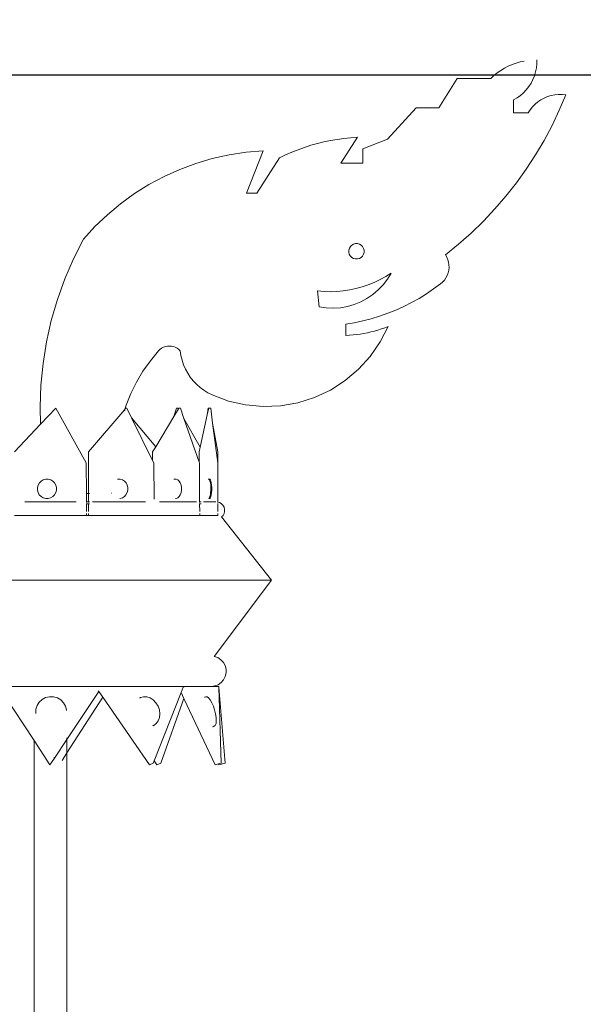
# Model space of a CAD drawing. Units: millimetres. Extents: x 7894 to 8038, y 6851 to 6951.
# Tile 11 of 49: x 7976.35 to 7978.394, y 6875.21 to 6878.784. Entities that reach past the tile are written whole.
import ezdxf

# ---------------------------------------------------------------- set-up
doc = ezdxf.new("R2010")
doc.units = ezdxf.units.MM
for name, color, linetype, lineweight in [('A-ANNO-DIMS', 2, 'Continuous', 18), ('A-FURN-ACCS', 8, 'Continuous', 13), ('A-FURN-SHLF', 7, 'Continuous', 30)]:
    doc.layers.add(name, color=color, linetype=linetype, lineweight=lineweight)
doc.styles.get("Standard").update_dxf_attribs({"font": 'arial.ttf'})
doc.dimstyles.new('ISO-25', dxfattribs={"dimtxt": 1, "dimasz": 1, "dimexe": 1.25, "dimexo": 0.625, "dimtad": 1, "dimdec": 0, "dimlunit": 4, "dimtxsty": 'Standard', "dimcen": 2.5, "dimclrt": 1, "dimadec": 0, "dimazin": 0, "dimtfac": 1, "dimtdec": 0, "dimtmove": 0, "dimatfit": 3, "dimfxl": 1, "dimarcsym": 0})

# ---------------------------------------------------------------- blocks, each defined once
blk = doc.blocks.new('*D36')
at = {"layer": 'A-ANNO-DIMS', "color": 0, "lineweight": -2, "transparency": 16777216}
for p, q in [((7980.8359, 6877.9586), (7980.8359, 6858.5122)), ((7944.4866, 6864.4359), (7944.4866, 6858.5122)), ((7945.4866, 6859.7622), (7979.8359, 6859.7622))]:
    blk.add_line(p, q, dxfattribs=at)
at = {"layer": 'A-ANNO-DIMS', "color": 0, "transparency": 16777216}
for points in [[(7945.4866, 6859.9288), (7945.4866, 6859.5955), (7944.4866, 6859.7622)], [(7979.8359, 6859.9288), (7979.8359, 6859.5955), (7980.8359, 6859.7622)]]:
    blk.add_solid(points, dxfattribs=at)
at = {"layer": 'Defpoints', "color": 0, "transparency": 16777216}
for p in [(7980.8359, 6878.5836), (7944.4866, 6865.0609), (7980.8359, 6859.7622)]:
    blk.add_point(p, dxfattribs=at)
at = {"layer": 'A-ANNO-DIMS', "color": 1, "transparency": 16777216, "insert": (7962.6613, 6860.9046), "char_height": 1, "attachment_point": 5}
blk.add_mtext('3\'-0 1/2"', dxfattribs=at)
blk = doc.blocks.new('*D39')
at = {"layer": 'A-ANNO-DIMS', "color": 0, "lineweight": -2, "transparency": 16777216}
for p, q in [((7982.6834, 6874.8578), (7982.6834, 6879.7661)), ((7964.1574, 6873.8578), (7983.9334, 6873.8578)), ((7982.6834, 6872.9028), (7982.6834, 6873.8578)), ((7981.4609, 6872.9028), (7983.9334, 6872.9028)), ((7982.6834, 6871.9028), (7982.6834, 6870.9028))]:
    blk.add_line(p, q, dxfattribs=at)
at = {"layer": 'A-ANNO-DIMS', "color": 0, "transparency": 16777216}
for points in [[(7982.5168, 6874.8578), (7982.8501, 6874.8578), (7982.6834, 6873.8578)], [(7982.5168, 6871.9028), (7982.8501, 6871.9028), (7982.6834, 6872.9028)]]:
    blk.add_solid(points, dxfattribs=at)
at = {"layer": 'Defpoints', "color": 0, "transparency": 16777216}
for p in [(7963.5324, 6873.8578), (7982.6834, 6873.8578), (7980.8359, 6872.9028)]:
    blk.add_point(p, dxfattribs=at)
at = {"layer": 'A-ANNO-DIMS', "color": 1, "transparency": 16777216, "insert": (7981.5479, 6877.8119), "char_height": 1, "attachment_point": 5, "rotation": 90}
blk.add_mtext('0\'-1"', dxfattribs=at)
blk = doc.blocks.new('*D40')
at = {"layer": 'A-ANNO-DIMS', "color": 0, "lineweight": -2, "transparency": 16777216}
for p, q in [((7982.6834, 6878.5836), (7982.6834, 6885.822)), ((7981.4609, 6878.5836), (7983.9334, 6878.5836)), ((7982.6834, 6874.8578), (7982.6834, 6877.5836)), ((7964.1574, 6873.8578), (7983.9334, 6873.8578))]:
    blk.add_line(p, q, dxfattribs=at)
at = {"layer": 'A-ANNO-DIMS', "color": 0, "transparency": 16777216}
for points in [[(7982.5168, 6877.5836), (7982.8501, 6877.5836), (7982.6834, 6878.5836)], [(7982.5168, 6874.8578), (7982.8501, 6874.8578), (7982.6834, 6873.8578)]]:
    blk.add_solid(points, dxfattribs=at)
at = {"layer": 'Defpoints', "color": 0, "transparency": 16777216}
for p in [(7980.8359, 6878.5836), (7982.6834, 6878.5836), (7963.5324, 6873.8578)]:
    blk.add_point(p, dxfattribs=at)
at = {"layer": 'A-ANNO-DIMS', "color": 1, "transparency": 16777216, "insert": (7981.5414, 6882.7028), "char_height": 1, "attachment_point": 5, "rotation": 90}
blk.add_mtext('0\'-4 1/2"', dxfattribs=at)

msp = doc.modelspace()

# ---------------------------------------------------------------- linework, layer by layer
at = {"layer": 'A-FURN-ACCS'}
for p, q in [((7978.1353, 6878.6211, 2.197), (7978.1497, 6878.6264, 2.197)), ((7978.1497, 6878.6264, 2.197), (7978.1645, 6878.6307, 2.197)), ((7978.1645, 6878.6307, 2.197), (7978.1795, 6878.6341, 2.197)), ((7978.2253, 6878.6385, 2.197), (7978.2252, 6878.6237, 2.197)), ((7978.0697, 6878.5816, 2.197), (7978.0818, 6878.5912, 2.197)), ((7978.0818, 6878.5912, 2.197), (7978.0944, 6878.5999, 2.197)), ((7978.0944, 6878.5999, 2.197), (7978.1076, 6878.6079, 2.197)), ((7978.1076, 6878.6079, 2.197), (7978.1212, 6878.6149, 2.197)), ((7978.1212, 6878.6149, 2.197), (7978.1353, 6878.6211, 2.197)), ((7978.2208, 6878.5946, 2.197), (7978.2166, 6878.5804, 2.197)), ((7978.2237, 6878.6091, 2.197), (7978.2208, 6878.5946, 2.197)), ((7978.2252, 6878.6237, 2.197), (7978.2237, 6878.6091, 2.197)), ((7977.8697, 6878.4643, 2.197), (7977.9359, 6878.5713, 2.197)), ((7977.9359, 6878.5713, 2.197), (7978.0583, 6878.5713, 2.197)), ((7978.0583, 6878.5713, 2.197), (7978.0697, 6878.5816, 2.197)), ((7978.2042, 6878.5537, 2.197), (7978.1962, 6878.5413, 2.197)), ((7978.211, 6878.5668, 2.197), (7978.2042, 6878.5537, 2.197)), ((7978.2166, 6878.5804, 2.197), (7978.211, 6878.5668, 2.197)), ((7978.1768, 6878.5191, 2.197), (7978.1656, 6878.5095, 2.197)), ((7978.187, 6878.5297, 2.197), (7978.1768, 6878.5191, 2.197)), ((7978.1962, 6878.5413, 2.197), (7978.187, 6878.5297, 2.197)), ((7978.1536, 6878.5009, 2.197), (7978.1408, 6878.4936, 2.197)), ((7978.1408, 6878.4936, 2.197), (7978.1408, 6878.4464, 2.197)), ((7978.1656, 6878.5095, 2.197), (7978.1536, 6878.5009, 2.197)), ((7978.2187, 6878.4773, 2.197), (7978.2291, 6878.4858, 2.197)), ((7978.2291, 6878.4858, 2.197), (7978.2402, 6878.4933, 2.197)), ((7978.2402, 6878.4933, 2.197), (7978.252, 6878.4997, 2.197)), ((7978.252, 6878.4997, 2.197), (7978.2644, 6878.5048, 2.197)), ((7978.2644, 6878.5048, 2.197), (7978.2772, 6878.5088, 2.197)), ((7978.2772, 6878.5088, 2.197), (7978.2903, 6878.5115, 2.197)), ((7978.2903, 6878.5115, 2.197), (7978.3036, 6878.513, 2.197)), ((7978.3036, 6878.513, 2.197), (7978.317, 6878.5131, 2.197)), ((7978.3304, 6878.5119, 2.197), (7978.3066, 6878.4554, 2.197)), ((7978.317, 6878.5131, 2.197), (7978.3304, 6878.5119, 2.197)), ((7977.6836, 6878.3509, 2.197), (7977.7876, 6878.4643, 2.197)), ((7977.7876, 6878.4643, 2.197), (7977.8697, 6878.4643, 2.197)), ((7978.1408, 6878.4464, 2.197), (7978.1932, 6878.4464, 2.197)), ((7978.1932, 6878.4464, 2.197), (7978.2007, 6878.4575, 2.197)), ((7978.2007, 6878.4575, 2.197), (7978.2092, 6878.4678, 2.197)), ((7978.2092, 6878.4678, 2.197), (7978.2187, 6878.4773, 2.197)), ((7978.3066, 6878.4554, 2.197), (7978.2803, 6878.4, 2.197)), ((7978.2803, 6878.4, 2.197), (7978.2515, 6878.3459, 2.197)), ((7977.4292, 6878.3349, 2.197), (7977.453, 6878.3408, 2.197)), ((7977.453, 6878.3408, 2.197), (7977.477, 6878.3458, 2.197)), ((7977.477, 6878.3458, 2.197), (7977.5011, 6878.3499, 2.197)), ((7977.5011, 6878.3499, 2.197), (7977.5254, 6878.3532, 2.197)), ((7977.5743, 6878.3572, 2.197), (7977.5139, 6878.263, 2.197)), ((7977.5254, 6878.3532, 2.197), (7977.5498, 6878.3556, 2.197)), ((7977.5498, 6878.3556, 2.197), (7977.5743, 6878.3572, 2.197)), ((7977.5943, 6878.3154, 2.197), (7977.6836, 6878.3509, 2.197)), ((7978.2515, 6878.3459, 2.197), (7978.2204, 6878.2931, 2.197)), ((7977.109, 6878.294, 2.197), (7977.1706, 6878.3034, 2.197)), ((7977.1706, 6878.3034, 2.197), (7977.2326, 6878.3087, 2.197)), ((7977.2326, 6878.3087, 2.197), (7977.1717, 6878.1542, 2.197)), ((7977.3142, 6878.2931, 2.197), (7977.3365, 6878.3031, 2.197)), ((7977.3365, 6878.3031, 2.197), (7977.3592, 6878.3123, 2.197)), ((7977.3592, 6878.3123, 2.197), (7977.3823, 6878.3206, 2.197)), ((7977.3823, 6878.3206, 2.197), (7977.4056, 6878.3282, 2.197)), ((7977.4056, 6878.3282, 2.197), (7977.4292, 6878.3349, 2.197)), ((7977.5943, 6878.263, 2.197), (7977.5943, 6878.3154, 2.197)), ((7976.9885, 6878.2626, 2.197), (7977.0482, 6878.2803, 2.197)), ((7977.0482, 6878.2803, 2.197), (7977.109, 6878.294, 2.197)), ((7977.2101, 6878.1542, 2.197), (7977.2921, 6878.2823, 2.197)), ((7977.2921, 6878.2823, 2.197), (7977.3142, 6878.2931, 2.197)), ((7978.2204, 6878.2931, 2.197), (7978.1869, 6878.2417, 2.197)), ((7976.8733, 6878.2153, 2.197), (7976.9301, 6878.2409, 2.197)), ((7976.9301, 6878.2409, 2.197), (7976.9885, 6878.2626, 2.197)), ((7977.5139, 6878.263, 2.197), (7977.5943, 6878.263, 2.197)), ((7978.1869, 6878.2417, 2.197), (7978.1512, 6878.1919, 2.197)), ((7976.8184, 6878.1858, 2.197), (7976.8733, 6878.2153, 2.197)), ((7976.7657, 6878.1527, 2.197), (7976.8184, 6878.1858, 2.197)), ((7978.1512, 6878.1919, 2.197), (7978.1132, 6878.1437, 2.197)), ((7976.7153, 6878.1161, 2.197), (7976.7657, 6878.1527, 2.197)), ((7977.1717, 6878.1542, 2.197), (7977.2101, 6878.1542, 2.197)), ((7978.1132, 6878.1437, 2.197), (7978.0732, 6878.0972, 2.197)), ((7976.6675, 6878.0762, 2.197), (7976.7153, 6878.1161, 2.197)), ((7978.0732, 6878.0972, 2.197), (7978.0312, 6878.0526, 2.197)), ((7976.6225, 6878.0331, 2.197), (7976.6675, 6878.0762, 2.197)), ((7976.5805, 6877.987, 2.197), (7976.6225, 6878.0331, 2.197)), ((7978.0312, 6878.0526, 2.197), (7977.9872, 6878.0099, 2.197)), ((7976.5805, 6877.987, 2.197), (7976.5447, 6877.9162, 2.197)), ((7977.9872, 6878.0099, 2.197), (7977.9413, 6877.9692, 2.197)), ((7977.5432, 6877.9399, 2.197), (7977.5433, 6877.9472, 2.197)), ((7977.5433, 6877.9472, 2.197), (7977.5452, 6877.9543, 2.197)), ((7977.5452, 6877.9543, 2.197), (7977.5489, 6877.9606, 2.197)), ((7977.5489, 6877.9606, 2.197), (7977.5541, 6877.9657, 2.197)), ((7977.5541, 6877.9657, 2.197), (7977.5604, 6877.9693, 2.197)), ((7977.5604, 6877.9693, 2.197), (7977.5675, 6877.9712, 2.197)), ((7977.5675, 6877.9712, 2.197), (7977.5748, 6877.9712, 2.197)), ((7977.5748, 6877.9712, 2.197), (7977.5818, 6877.9692, 2.197)), ((7977.5818, 6877.9692, 2.197), (7977.5881, 6877.9656, 2.197)), ((7977.5881, 6877.9656, 2.197), (7977.5933, 6877.9604, 2.197)), ((7977.5933, 6877.9604, 2.197), (7977.5969, 6877.954, 2.197)), ((7977.5969, 6877.954, 2.197), (7977.5987, 6877.947, 2.197)), ((7977.5987, 6877.947, 2.197), (7977.5987, 6877.9397, 2.197)), ((7977.9413, 6877.9692, 2.197), (7977.8937, 6877.9306, 2.197)), ((7976.5447, 6877.9162, 2.197), (7976.5133, 6877.8432, 2.197)), ((7977.5451, 6877.9329, 2.197), (7977.5432, 6877.9399, 2.197)), ((7977.5487, 6877.9265, 2.197), (7977.5451, 6877.9329, 2.197)), ((7977.5538, 6877.9214, 2.197), (7977.5487, 6877.9265, 2.197)), ((7977.5601, 6877.9177, 2.197), (7977.5538, 6877.9214, 2.197)), ((7977.5672, 6877.9158, 2.197), (7977.5601, 6877.9177, 2.197)), ((7977.5745, 6877.9157, 2.197), (7977.5672, 6877.9158, 2.197)), ((7977.5815, 6877.9176, 2.197), (7977.5745, 6877.9157, 2.197)), ((7977.5879, 6877.9212, 2.197), (7977.5815, 6877.9176, 2.197)), ((7977.5931, 6877.9263, 2.197), (7977.5879, 6877.9212, 2.197)), ((7977.5968, 6877.9326, 2.197), (7977.5931, 6877.9263, 2.197)), ((7977.5987, 6877.9397, 2.197), (7977.5968, 6877.9326, 2.197)), ((7977.8937, 6877.9306, 2.197), (7977.8985, 6877.9222, 2.197)), ((7977.8985, 6877.9222, 2.197), (7977.9023, 6877.9131, 2.197)), ((7977.9023, 6877.9131, 2.197), (7977.9049, 6877.9037, 2.197)), ((7977.9056, 6877.8746, 2.197), (7977.9034, 6877.8651, 2.197)), ((7977.9049, 6877.9037, 2.197), (7977.9064, 6877.8941, 2.197)), ((7977.9066, 6877.8843, 2.197), (7977.9056, 6877.8746, 2.197)), ((7977.9064, 6877.8941, 2.197), (7977.9066, 6877.8843, 2.197)), ((7976.5133, 6877.8432, 2.197), (7976.4865, 6877.7684, 2.197)), ((7977.6566, 6877.8406, 2.197), (7977.6355, 6877.8306, 2.197)), ((7977.677, 6877.8518, 2.197), (7977.6566, 6877.8406, 2.197)), ((7977.6833, 6877.8424, 2.197), (7977.6676, 6877.822, 2.197)), ((7977.6968, 6877.8643, 2.197), (7977.677, 6877.8518, 2.197)), ((7977.6968, 6877.8643, 2.197), (7977.6833, 6877.8424, 2.197)), ((7977.89, 6877.8392, 2.197), (7977.8835, 6877.8319, 2.197)), ((7977.8955, 6877.8472, 2.197), (7977.89, 6877.8392, 2.197)), ((7977.9, 6877.8559, 2.197), (7977.8955, 6877.8472, 2.197)), ((7977.9034, 6877.8651, 2.197), (7977.9, 6877.8559, 2.197)), ((7977.5464, 6877.8033, 2.197), (7977.5233, 6877.7998, 2.197)), ((7977.5692, 6877.8081, 2.197), (7977.5464, 6877.8033, 2.197)), ((7977.5917, 6877.8143, 2.197), (7977.5692, 6877.8081, 2.197)), ((7977.6138, 6877.8218, 2.197), (7977.5917, 6877.8143, 2.197)), ((7977.6355, 6877.8306, 2.197), (7977.6138, 6877.8218, 2.197)), ((7977.6499, 6877.8034, 2.197), (7977.6303, 6877.7868, 2.197)), ((7977.6676, 6877.822, 2.197), (7977.6499, 6877.8034, 2.197)), ((7977.8508, 6877.8068, 2.197), (7977.8246, 6877.7892, 2.197)), ((7977.8761, 6877.8255, 2.197), (7977.8508, 6877.8068, 2.197)), ((7977.8835, 6877.8319, 2.197), (7977.8761, 6877.8255, 2.197)), ((7976.4865, 6877.7684, 2.197), (7976.4643, 6877.6922, 2.197)), ((7977.4534, 6877.7975, 2.197), (7977.4301, 6877.7995, 2.197)), ((7977.4301, 6877.7995, 2.197), (7977.4358, 6877.7415, 2.197)), ((7977.4767, 6877.7969, 2.197), (7977.4534, 6877.7975, 2.197)), ((7977.5, 6877.7977, 2.197), (7977.4767, 6877.7969, 2.197)), ((7977.5233, 6877.7998, 2.197), (7977.5, 6877.7977, 2.197)), ((7977.6091, 6877.7723, 2.197), (7977.5864, 6877.7602, 2.197)), ((7977.6303, 6877.7868, 2.197), (7977.6091, 6877.7723, 2.197)), ((7977.7978, 6877.7727, 2.197), (7977.7703, 6877.7573, 2.197)), ((7977.8246, 6877.7892, 2.197), (7977.7978, 6877.7727, 2.197)), ((7977.4613, 6877.7379, 2.197), (7977.4358, 6877.7415, 2.197)), ((7977.487, 6877.737, 2.197), (7977.4613, 6877.7379, 2.197)), ((7977.5126, 6877.7388, 2.197), (7977.487, 6877.737, 2.197)), ((7977.5379, 6877.7433, 2.197), (7977.5126, 6877.7388, 2.197)), ((7977.5626, 6877.7505, 2.197), (7977.5379, 6877.7433, 2.197)), ((7977.5864, 6877.7602, 2.197), (7977.5626, 6877.7505, 2.197)), ((7977.7422, 6877.7432, 2.197), (7977.7135, 6877.7302, 2.197)), ((7977.7703, 6877.7573, 2.197), (7977.7422, 6877.7432, 2.197)), ((7977.6244, 6877.6986, 2.197), (7977.594, 6877.6906, 2.197)), ((7977.6546, 6877.7079, 2.197), (7977.6244, 6877.6986, 2.197)), ((7977.6842, 6877.7184, 2.197), (7977.6546, 6877.7079, 2.197)), ((7977.7135, 6877.7302, 2.197), (7977.6842, 6877.7184, 2.197)), ((7976.4643, 6877.6922, 2.197), (7976.4469, 6877.6147, 2.197)), ((7977.5632, 6877.6839, 2.197), (7977.5322, 6877.6784, 2.197)), ((7977.5322, 6877.6784, 2.197), (7977.5322, 6877.6382, 2.197)), ((7977.594, 6877.6906, 2.197), (7977.5632, 6877.6839, 2.197)), ((7977.6488, 6877.6576, 2.197), (7977.6614, 6877.6617, 2.197)), ((7977.6861, 6877.6709, 2.197), (7977.6571, 6877.6143, 2.197)), ((7977.6614, 6877.6617, 2.197), (7977.6738, 6877.6661, 2.197)), ((7977.6738, 6877.6661, 2.197), (7977.6861, 6877.6709, 2.197)), ((7977.5322, 6877.6382, 2.197), (7977.5453, 6877.6389, 2.197)), ((7977.5453, 6877.6389, 2.197), (7977.5585, 6877.6399, 2.197)), ((7977.5585, 6877.6399, 2.197), (7977.5716, 6877.6412, 2.197)), ((7977.5716, 6877.6412, 2.197), (7977.5846, 6877.643, 2.197)), ((7977.5846, 6877.643, 2.197), (7977.5976, 6877.6452, 2.197)), ((7977.5976, 6877.6452, 2.197), (7977.6106, 6877.6477, 2.197)), ((7977.6106, 6877.6477, 2.197), (7977.6234, 6877.6506, 2.197)), ((7977.6234, 6877.6506, 2.197), (7977.6362, 6877.6539, 2.197)), ((7977.6362, 6877.6539, 2.197), (7977.6488, 6877.6576, 2.197)), ((7976.4469, 6877.6147, 2.197), (7976.4343, 6877.5362, 2.197)), ((7976.8644, 6877.5915, 2.197), (7976.8584, 6877.5872, 2.197)), ((7976.8709, 6877.595, 2.197), (7976.8644, 6877.5915, 2.197)), ((7976.8779, 6877.5975, 2.197), (7976.8709, 6877.595, 2.197)), ((7976.8851, 6877.599, 2.197), (7976.8779, 6877.5975, 2.197)), ((7976.8924, 6877.5996, 2.197), (7976.8851, 6877.599, 2.197)), ((7976.8998, 6877.599, 2.197), (7976.8924, 6877.5996, 2.197)), ((7976.907, 6877.5975, 2.197), (7976.8998, 6877.599, 2.197)), ((7976.914, 6877.595, 2.197), (7976.907, 6877.5975, 2.197)), ((7976.9205, 6877.5915, 2.197), (7976.914, 6877.595, 2.197)), ((7976.9264, 6877.5872, 2.197), (7976.9205, 6877.5915, 2.197)), ((7977.6571, 6877.6143, 2.197), (7977.621, 6877.5621, 2.197)), ((7976.8531, 6877.5821, 2.197), (7976.8235, 6877.5465, 2.197)), ((7976.8584, 6877.5872, 2.197), (7976.8531, 6877.5821, 2.197)), ((7976.9318, 6877.5821, 2.197), (7976.9264, 6877.5872, 2.197)), ((7976.9343, 6877.565, 2.197), (7976.9318, 6877.5821, 2.197)), ((7976.9383, 6877.5483, 2.197), (7976.9343, 6877.565, 2.197)), ((7977.621, 6877.5621, 2.197), (7977.5784, 6877.5151, 2.197)), ((7976.4343, 6877.5362, 2.197), (7976.4266, 6877.4572, 2.197)), ((7976.8235, 6877.5465, 2.197), (7976.7968, 6877.5088, 2.197)), ((7976.9438, 6877.5319, 2.197), (7976.9383, 6877.5483, 2.197)), ((7976.9506, 6877.5161, 2.197), (7976.9438, 6877.5319, 2.197)), ((7976.7968, 6877.5088, 2.197), (7976.7731, 6877.469, 2.197)), ((7976.9588, 6877.501, 2.197), (7976.9506, 6877.5161, 2.197)), ((7976.9683, 6877.4866, 2.197), (7976.9588, 6877.501, 2.197)), ((7976.979, 6877.4731, 2.197), (7976.9683, 6877.4866, 2.197)), ((7977.5784, 6877.5151, 2.197), (7977.5299, 6877.4741, 2.197)), ((7976.4266, 6877.4572, 2.197), (7976.4238, 6877.3778, 2.197)), ((7976.7731, 6877.469, 2.197), (7976.7526, 6877.4275, 2.197)), ((7976.9909, 6877.4606, 2.197), (7976.979, 6877.4731, 2.197)), ((7977.0038, 6877.4492, 2.197), (7976.9909, 6877.4606, 2.197)), ((7977.0176, 6877.4389, 2.197), (7977.0038, 6877.4492, 2.197)), ((7977.5299, 6877.4741, 2.197), (7977.4764, 6877.4399, 2.197)), ((7976.7526, 6877.4275, 2.197), (7976.7355, 6877.3845, 2.197)), ((7977.0323, 6877.4299, 2.197), (7977.0176, 6877.4389, 2.197)), ((7977.0477, 6877.4222, 2.197), (7977.0323, 6877.4299, 2.197)), ((7977.1072, 6877.4001, 2.197), (7977.0477, 6877.4222, 2.197)), ((7977.4189, 6877.413, 2.197), (7977.3583, 6877.3939, 2.197)), ((7977.4764, 6877.4399, 2.197), (7977.4189, 6877.413, 2.197)), ((7976.4238, 6877.3778, 2.197), (7976.4254, 6877.3158, 2.197)), ((7976.4811, 6877.3745, 2.197), (7976.4254, 6877.3158, 2.197)), ((7976.5903, 6877.1753, 2.197), (7976.4811, 6877.3745, 2.197)), ((7976.7355, 6877.3845, 2.197), (7976.7311, 6877.3702, 2.197)), ((7976.7348, 6877.3745, 2.197), (7976.7311, 6877.3702, 2.197)), ((7976.7348, 6877.3745, 2.197), (7976.7379, 6877.3745, 2.197)), ((7976.7552, 6877.3393, 2.197), (7976.7379, 6877.3745, 2.197)), ((7976.9082, 6877.3433, 2.197), (7976.9184, 6877.3745, 2.197)), ((7976.9184, 6877.3745, 2.197), (7976.924, 6877.3745, 2.197)), ((7976.924, 6877.3745, 2.197), (7976.9254, 6877.3721, 2.197)), ((7976.9269, 6877.3745, 2.197), (7976.9254, 6877.3721, 2.197)), ((7976.9269, 6877.3745, 2.197), (7976.9323, 6877.3745, 2.197)), ((7976.9454, 6877.3369, 2.197), (7976.9323, 6877.3745, 2.197)), ((7977.03, 6877.3496, 2.197), (7977.0326, 6877.3745, 2.197)), ((7977.0355, 6877.3745, 2.197), (7977.03, 6877.3496, 2.197)), ((7977.0326, 6877.3745, 2.197), (7977.0355, 6877.3745, 2.197)), ((7977.0355, 6877.3745, 2.197), (7977.0423, 6877.3745, 2.197)), ((7977.0423, 6877.3745, 2.197), (7977.0492, 6877.3201, 2.197)), ((7977.1691, 6877.3861, 2.197), (7977.1072, 6877.4001, 2.197)), ((7977.2324, 6877.3803, 2.197), (7977.1691, 6877.3861, 2.197)), ((7977.2958, 6877.3829, 2.197), (7977.2324, 6877.3803, 2.197)), ((7977.3583, 6877.3939, 2.197), (7977.2958, 6877.3829, 2.197)), ((7976.7307, 6877.3688, 2.197), (7976.5997, 6877.2159, 2.197)), ((7976.7307, 6877.3688, 2.197), (7976.7293, 6877.3645, 2.197)), ((7976.7311, 6877.3702, 2.197), (7976.7307, 6877.3688, 2.197)), ((7976.7307, 6877.3688, 2.197), (7976.7318, 6877.3674, 2.197)), ((7976.7552, 6877.3393, 2.197), (7976.8428, 6877.2342, 2.197)), ((7976.7552, 6877.3393, 2.197), (7976.8318, 6877.1842, 2.197)), ((7976.9082, 6877.3433, 2.197), (7976.8428, 6877.2342, 2.197)), ((7976.9254, 6877.3721, 2.197), (7976.9082, 6877.3433, 2.197)), ((7977.03, 6877.3496, 2.197), (7977.0044, 6877.2329, 2.197)), ((7976.4254, 6877.3158, 2.197), (7976.3309, 6877.2159, 2.197)), ((7976.9454, 6877.3369, 2.197), (7977.0044, 6877.2329, 2.197)), ((7976.9454, 6877.3369, 2.197), (7977.0007, 6877.1778, 2.197)), ((7977.0492, 6877.3201, 2.197), (7977.0679, 6877.2159, 2.197)), ((7977.0676, 6877.1753, 2.197), (7977.0492, 6877.3201, 2.197)), ((7976.8428, 6877.2342, 2.197), (7976.8318, 6877.2159, 2.197)), ((7977.0044, 6877.2329, 2.197), (7977.0007, 6877.2159, 2.197)), ((7976.5997, 6877.2159, 2.197), (7976.5997, 6877.0643, 2.197)), ((7976.8318, 6877.2159, 2.197), (7976.8318, 6877.1842, 2.197)), ((7977.0007, 6877.2159, 2.197), (7977.0007, 6877.1778, 2.197)), ((7977.0679, 6877.2159, 2.197), (7977.0676, 6877.1753, 2.197)), ((7976.5903, 6877.1753, 2.197), (7976.5913, 6877.0642, 2.197)), ((7976.8362, 6877.1753, 2.197), (7976.8318, 6877.1842, 2.197)), ((7976.8362, 6877.1753, 2.197), (7976.8372, 6877.0442, 2.197)), ((7977.0015, 6877.1753, 2.197), (7977.0007, 6877.1778, 2.197)), ((7977.0015, 6877.1753, 2.197), (7977.0023, 6877.0335, 2.197)), ((7977.0676, 6877.1753, 2.197), (7977.0679, 6877.033, 2.197)), ((7976.414, 6877.086, 2.197), (7976.4164, 6877.0948, 2.197)), ((7976.4164, 6877.0948, 2.197), (7976.421, 6877.1027, 2.197)), ((7976.421, 6877.1027, 2.197), (7976.4274, 6877.1091, 2.197)), ((7976.4274, 6877.1091, 2.197), (7976.4353, 6877.1137, 2.197)), ((7976.4353, 6877.1137, 2.197), (7976.4442, 6877.116, 2.197)), ((7976.4442, 6877.116, 2.197), (7976.4533, 6877.116, 2.197)), ((7976.4533, 6877.116, 2.197), (7976.4621, 6877.1136, 2.197)), ((7976.4621, 6877.1136, 2.197), (7976.47, 6877.109, 2.197)), ((7976.47, 6877.109, 2.197), (7976.4764, 6877.1025, 2.197)), ((7976.4764, 6877.1025, 2.197), (7976.481, 6877.0946, 2.197)), ((7976.481, 6877.0946, 2.197), (7976.4833, 6877.0858, 2.197)), ((7976.7047, 6877.116, 2.197), (7976.7062, 6877.116, 2.197)), ((7976.7062, 6877.116, 2.197), (7976.7144, 6877.116, 2.197)), ((7976.7144, 6877.116, 2.197), (7976.7223, 6877.1136, 2.197)), ((7976.7223, 6877.1136, 2.197), (7976.7294, 6877.109, 2.197)), ((7976.7294, 6877.109, 2.197), (7976.7352, 6877.1025, 2.197)), ((7976.7352, 6877.1025, 2.197), (7976.7393, 6877.0946, 2.197)), ((7976.7393, 6877.0946, 2.197), (7976.7414, 6877.0858, 2.197)), ((7976.9089, 6877.116, 2.197), (7976.9117, 6877.116, 2.197)), ((7976.9117, 6877.116, 2.197), (7976.9174, 6877.116, 2.197)), ((7976.9174, 6877.116, 2.197), (7976.923, 6877.1136, 2.197)), ((7976.923, 6877.1136, 2.197), (7976.928, 6877.109, 2.197)), ((7976.928, 6877.109, 2.197), (7976.9321, 6877.1025, 2.197)), ((7976.9321, 6877.1025, 2.197), (7976.935, 6877.0946, 2.197)), ((7976.935, 6877.0946, 2.197), (7976.9364, 6877.0858, 2.197)), ((7977.0337, 6877.116, 2.197), (7977.0358, 6877.116, 2.197)), ((7977.0358, 6877.116, 2.197), (7977.0379, 6877.1136, 2.197)), ((7977.0358, 6877.116, 2.197), (7977.0371, 6877.116, 2.197)), ((7977.0371, 6877.116, 2.197), (7977.0392, 6877.116, 2.197)), ((7977.0379, 6877.1136, 2.197), (7977.0397, 6877.109, 2.197)), ((7977.0392, 6877.116, 2.197), (7977.0413, 6877.1136, 2.197)), ((7977.0397, 6877.109, 2.197), (7977.0412, 6877.1025, 2.197)), ((7977.0412, 6877.1025, 2.197), (7977.0423, 6877.0946, 2.197)), ((7977.0413, 6877.1136, 2.197), (7977.0431, 6877.109, 2.197)), ((7977.0423, 6877.0946, 2.197), (7977.0428, 6877.0858, 2.197)), ((7977.0431, 6877.109, 2.197), (7977.0446, 6877.1025, 2.197)), ((7977.0446, 6877.1025, 2.197), (7977.0457, 6877.0946, 2.197)), ((7977.0457, 6877.0946, 2.197), (7977.0462, 6877.0858, 2.197)), ((7976.414, 6877.0769, 2.197), (7976.414, 6877.086, 2.197)), ((7976.4163, 6877.0681, 2.197), (7976.414, 6877.0769, 2.197)), ((7976.4208, 6877.0601, 2.197), (7976.4163, 6877.0681, 2.197)), ((7976.4273, 6877.0537, 2.197), (7976.4208, 6877.0601, 2.197)), ((7976.4352, 6877.0491, 2.197), (7976.4273, 6877.0537, 2.197)), ((7976.4698, 6877.0536, 2.197), (7976.4619, 6877.049, 2.197)), ((7976.4763, 6877.06, 2.197), (7976.4698, 6877.0536, 2.197)), ((7976.4809, 6877.0679, 2.197), (7976.4763, 6877.06, 2.197)), ((7976.4833, 6877.0767, 2.197), (7976.4809, 6877.0679, 2.197)), ((7976.4833, 6877.0858, 2.197), (7976.4833, 6877.0767, 2.197)), ((7976.5997, 6877.0643, 2.197), (7976.5913, 6877.0642, 2.197)), ((7976.5913, 6877.0642, 2.197), (7976.5916, 6877.0335, 2.197)), ((7976.6028, 6877.0643, 2.197), (7976.5997, 6877.0643, 2.197)), ((7976.5997, 6877.0643, 2.197), (7976.5997, 6877.0335, 2.197)), ((7976.6827, 6877.065, 2.197), (7976.6812, 6877.065, 2.197)), ((7976.7293, 6877.0536, 2.197), (7976.7222, 6877.049, 2.197)), ((7976.7351, 6877.06, 2.197), (7976.7293, 6877.0536, 2.197)), ((7976.7392, 6877.0679, 2.197), (7976.7351, 6877.06, 2.197)), ((7976.7414, 6877.0767, 2.197), (7976.7392, 6877.0679, 2.197)), ((7976.7414, 6877.0858, 2.197), (7976.7414, 6877.0767, 2.197)), ((7976.9279, 6877.0536, 2.197), (7976.9229, 6877.049, 2.197)), ((7976.932, 6877.06, 2.197), (7976.9279, 6877.0536, 2.197)), ((7976.9349, 6877.0679, 2.197), (7976.932, 6877.06, 2.197)), ((7976.9364, 6877.0767, 2.197), (7976.9349, 6877.0679, 2.197)), ((7976.9364, 6877.0858, 2.197), (7976.9364, 6877.0767, 2.197)), ((7977.0397, 6877.0536, 2.197), (7977.0378, 6877.049, 2.197)), ((7977.0412, 6877.06, 2.197), (7977.0397, 6877.0536, 2.197)), ((7977.0422, 6877.0679, 2.197), (7977.0412, 6877.06, 2.197)), ((7977.0431, 6877.0536, 2.197), (7977.0412, 6877.049, 2.197)), ((7977.0428, 6877.0767, 2.197), (7977.0422, 6877.0679, 2.197)), ((7977.0428, 6877.0858, 2.197), (7977.0428, 6877.0767, 2.197)), ((7977.0446, 6877.06, 2.197), (7977.0431, 6877.0536, 2.197)), ((7977.0456, 6877.0679, 2.197), (7977.0446, 6877.06, 2.197)), ((7977.0462, 6877.0767, 2.197), (7977.0456, 6877.0679, 2.197)), ((7977.0462, 6877.0858, 2.197), (7977.0462, 6877.0767, 2.197)), ((7976.3685, 6877.0335, 2.197), (7976.5544, 6877.0335, 2.197)), ((7976.444, 6877.0467, 2.197), (7976.4352, 6877.0491, 2.197)), ((7976.4531, 6877.0467, 2.197), (7976.444, 6877.0467, 2.197)), ((7976.4619, 6877.049, 2.197), (7976.4531, 6877.0467, 2.197)), ((7976.5916, 6877.0335, 2.197), (7976.5916, 6877.0315, 2.197)), ((7976.5997, 6877.0335, 2.197), (7976.5916, 6877.0335, 2.197)), ((7976.5916, 6877.0276, 2.197), (7976.5916, 6877.0271, 2.197)), ((7976.5916, 6877.0271, 2.197), (7976.5918, 6876.9995, 2.197)), ((7976.5997, 6877.0271, 2.197), (7976.5916, 6877.0271, 2.197)), ((7976.6028, 6877.0335, 2.197), (7976.5997, 6877.0335, 2.197)), ((7976.5997, 6877.0335, 2.197), (7976.5997, 6877.0315, 2.197)), ((7976.5997, 6877.0276, 2.197), (7976.5997, 6877.0271, 2.197)), ((7976.6028, 6877.0271, 2.197), (7976.5997, 6877.0271, 2.197)), ((7976.5997, 6877.0271, 2.197), (7976.5997, 6876.9995, 2.197)), ((7976.6137, 6877.0335, 2.197), (7976.8059, 6877.0335, 2.197)), ((7976.7127, 6877.0467, 2.197), (7976.7142, 6877.0467, 2.197)), ((7976.7222, 6877.049, 2.197), (7976.7142, 6877.0467, 2.197)), ((7976.9908, 6877.0335, 2.197), (7976.8569, 6877.0335, 2.197)), ((7976.9146, 6877.0467, 2.197), (7976.9173, 6877.0467, 2.197)), ((7976.9229, 6877.049, 2.197), (7976.9173, 6877.0467, 2.197)), ((7977.0075, 6877.0335, 2.197), (7977.0023, 6877.0335, 2.197)), ((7977.0023, 6877.0335, 2.197), (7977.0023, 6877.0315, 2.197)), ((7977.0023, 6877.0276, 2.197), (7977.0023, 6877.0271, 2.197)), ((7977.0075, 6877.0271, 2.197), (7977.0023, 6877.0271, 2.197)), ((7977.0023, 6877.0271, 2.197), (7977.0025, 6876.9995, 2.197)), ((7977.0165, 6877.0335, 2.197), (7977.0607, 6877.0335, 2.197)), ((7977.0378, 6877.049, 2.197), (7977.0358, 6877.0467, 2.197)), ((7977.0358, 6877.0467, 2.197), (7977.0392, 6877.0467, 2.197)), ((7977.0412, 6877.049, 2.197), (7977.0392, 6877.0467, 2.197)), ((7977.0679, 6877.033, 2.197), (7977.0738, 6877.0315, 2.197)), ((7977.0679, 6877.033, 2.197), (7977.0679, 6877.0315, 2.197)), ((7977.0679, 6877.0276, 2.197), (7977.0679, 6876.9995, 2.197)), ((7977.0738, 6877.0315, 2.197), (7977.0808, 6877.0276, 2.197)), ((7977.0808, 6877.0276, 2.197), (7977.0865, 6877.0221, 2.197)), ((7977.0865, 6877.0221, 2.197), (7977.0906, 6877.0152, 2.197)), ((7976.3309, 6876.9848, 2.197), (7976.592, 6876.9848, 2.197)), ((7976.5919, 6876.9918, 2.197), (7976.592, 6876.9848, 2.197)), ((7976.5997, 6876.9848, 2.197), (7976.592, 6876.9848, 2.197)), ((7976.5997, 6876.9918, 2.197), (7976.5997, 6876.9848, 2.197)), ((7977.0026, 6876.9848, 2.197), (7976.5997, 6876.9848, 2.197)), ((7977.0025, 6876.9918, 2.197), (7977.0026, 6876.9848, 2.197)), ((7977.0679, 6876.9848, 2.197), (7977.0026, 6876.9848, 2.197)), ((7977.0679, 6876.9918, 2.197), (7977.0679, 6876.9848, 2.197)), ((7977.0871, 6876.9848, 2.197), (7977.0815, 6876.9791, 2.197)), ((7977.091, 6876.9918, 2.197), (7977.0871, 6876.9848, 2.197)), ((7977.0906, 6877.0152, 2.197), (7977.0928, 6877.0075, 2.197)), ((7977.0929, 6876.9995, 2.197), (7977.091, 6876.9918, 2.197)), ((7977.0928, 6877.0075, 2.197), (7977.0929, 6876.9995, 2.197)), ((7977.0815, 6876.9791, 2.197), (7977.2625, 6876.7501, 2.197)), ((7977.2625, 6876.7501, 2.197), (7975.6603, 6876.7501, 2.197)), ((7977.2625, 6876.7501, 2.197), (7977.0553, 6876.4729, 2.197)), ((7977.0553, 6876.4729, 2.197), (7977.068, 6876.4685, 2.197)), ((7977.068, 6876.4685, 2.197), (7977.0792, 6876.4611, 2.197)), ((7977.0792, 6876.4611, 2.197), (7977.0883, 6876.4513, 2.197)), ((7977.0883, 6876.4513, 2.197), (7977.0947, 6876.4395, 2.197)), ((7977.0947, 6876.4395, 2.197), (7977.0982, 6876.4266, 2.197)), ((7977.0983, 6876.4132, 2.197), (7977.0953, 6876.4001, 2.197)), ((7977.0982, 6876.4266, 2.197), (7977.0983, 6876.4132, 2.197)), ((7977.0804, 6876.3781, 2.197), (7977.0694, 6876.3704, 2.197)), ((7977.0892, 6876.3882, 2.197), (7977.0804, 6876.3781, 2.197)), ((7977.0953, 6876.4001, 2.197), (7977.0892, 6876.3882, 2.197)), ((7976.6121, 6876.364, 2.197), (7976.2778, 6876.364, 2.197)), ((7976.5208, 6876.1711, 2.197), (7976.6369, 6876.3454, 2.197)), ((7976.6413, 6876.3637, 2.197), (7976.6121, 6876.364, 2.197)), ((7976.6369, 6876.3454, 2.197), (7976.6347, 6876.3485, 2.197)), ((7976.6506, 6876.3255, 2.197), (7976.6369, 6876.3454, 2.197)), ((7976.6413, 6876.3637, 2.197), (7976.6419, 6876.364, 2.197)), ((7976.6419, 6876.364, 2.197), (7976.6433, 6876.364, 2.197)), ((7976.9439, 6876.364, 2.197), (7976.6433, 6876.364, 2.197)), ((7976.8372, 6876.094, 2.197), (7976.9351, 6876.3421, 2.197)), ((7976.9351, 6876.3421, 2.197), (7976.943, 6876.3619, 2.197)), ((7976.9453, 6876.3203, 2.197), (7976.9351, 6876.3421, 2.197)), ((7976.943, 6876.3619, 2.197), (7976.9502, 6876.364, 2.197)), ((7976.943, 6876.3619, 2.197), (7976.9439, 6876.364, 2.197)), ((7976.9439, 6876.364, 2.197), (7976.9502, 6876.364, 2.197)), ((7976.9502, 6876.364, 2.197), (7977.0436, 6876.364, 2.197)), ((7977.0569, 6876.3656, 2.197), (7977.0436, 6876.364, 2.197)), ((7977.0704, 6876.3637, 2.197), (7977.0436, 6876.364, 2.197)), ((7977.0694, 6876.3704, 2.197), (7977.0569, 6876.3656, 2.197)), ((7977.0714, 6876.364, 2.197), (7977.0704, 6876.3637, 2.197)), ((7977.0716, 6876.3616, 2.197), (7977.0714, 6876.364, 2.197)), ((7977.0952, 6876.0853, 2.197), (7977.0716, 6876.3616, 2.197)), ((7977.0807, 6876.0853, 2.197), (7977.0716, 6876.3616, 2.197)), ((7976.402, 6876.1672, 2.197), (7976.2926, 6876.335, 2.197)), ((7976.4124, 6876.295, 2.197), (7976.42, 6876.3071, 2.197)), ((7976.42, 6876.3071, 2.197), (7976.4306, 6876.3167, 2.197)), ((7976.4306, 6876.3167, 2.197), (7976.4435, 6876.3234, 2.197)), ((7976.4435, 6876.3234, 2.197), (7976.4577, 6876.3267, 2.197)), ((7976.4577, 6876.3267, 2.197), (7976.4723, 6876.3263, 2.197)), ((7976.4723, 6876.3263, 2.197), (7976.4863, 6876.3223, 2.197)), ((7976.4863, 6876.3223, 2.197), (7976.4987, 6876.3149, 2.197)), ((7976.4987, 6876.3149, 2.197), (7976.5087, 6876.3046, 2.197)), ((7976.5087, 6876.3046, 2.197), (7976.5157, 6876.2922, 2.197)), ((7976.5208, 6876.1224, 2.197), (7976.6506, 6876.3255, 2.197)), ((7976.8203, 6876.079, 2.197), (7976.6506, 6876.3255, 2.197)), ((7976.7845, 6876.3221, 2.197), (7976.7861, 6876.3226, 2.197)), ((7976.7861, 6876.3226, 2.197), (7976.7873, 6876.3234, 2.197)), ((7976.7873, 6876.3234, 2.197), (7976.7985, 6876.3267, 2.197)), ((7976.7985, 6876.3267, 2.197), (7976.8106, 6876.3263, 2.197)), ((7976.8106, 6876.3263, 2.197), (7976.8227, 6876.3223, 2.197)), ((7976.8227, 6876.3223, 2.197), (7976.834, 6876.3149, 2.197)), ((7976.834, 6876.3149, 2.197), (7976.8439, 6876.3046, 2.197)), ((7976.8439, 6876.3046, 2.197), (7976.8515, 6876.2922, 2.197)), ((7976.8619, 6876.0853, 2.197), (7976.9453, 6876.3203, 2.197)), ((7977.0584, 6876.079, 2.197), (7976.9453, 6876.3203, 2.197)), ((7977.0194, 6876.3254, 2.197), (7977.0242, 6876.3267, 2.197)), ((7977.0194, 6876.3254, 2.197), (7977.0223, 6876.3251, 2.197)), ((7977.0242, 6876.3267, 2.197), (7977.0291, 6876.3263, 2.197)), ((7977.0291, 6876.3263, 2.197), (7977.0347, 6876.3223, 2.197)), ((7977.0347, 6876.3223, 2.197), (7977.0407, 6876.3149, 2.197)), ((7977.0407, 6876.3149, 2.197), (7977.0466, 6876.3046, 2.197)), ((7977.0466, 6876.3046, 2.197), (7977.052, 6876.2922, 2.197)), ((7976.4078, 6876.2673, 2.197), (7976.4082, 6876.2815, 2.197)), ((7976.4078, 6876.2661, 2.197), (7976.4078, 6876.2673, 2.197)), ((7976.4082, 6876.2815, 2.197), (7976.4124, 6876.295, 2.197)), ((7976.5157, 6876.2922, 2.197), (7976.519, 6876.2785, 2.197)), ((7976.519, 6876.2772, 2.197), (7976.519, 6876.2785, 2.197)), ((7976.8515, 6876.2922, 2.197), (7976.8563, 6876.2785, 2.197)), ((7976.8563, 6876.2785, 2.197), (7976.8581, 6876.2644, 2.197)), ((7977.052, 6876.2922, 2.197), (7977.0566, 6876.2785, 2.197)), ((7977.0566, 6876.2785, 2.197), (7977.0601, 6876.2644, 2.197)), ((7976.8523, 6876.2389, 2.197), (7976.8451, 6876.2292, 2.197)), ((7976.8568, 6876.2509, 2.197), (7976.8523, 6876.2389, 2.197)), ((7976.8581, 6876.2644, 2.197), (7976.8568, 6876.2509, 2.197)), ((7977.0601, 6876.2644, 2.197), (7977.0621, 6876.2509, 2.197)), ((7977.0626, 6876.2389, 2.197), (7977.0616, 6876.2292, 2.197)), ((7977.0621, 6876.2509, 2.197), (7977.0626, 6876.2389, 2.197)), ((7976.8339, 6876.222, 2.197), (7976.8326, 6876.2211, 2.197)), ((7976.8339, 6876.222, 2.197), (7976.8355, 6876.2225, 2.197)), ((7976.8451, 6876.2292, 2.197), (7976.8355, 6876.2225, 2.197)), ((7977.0522, 6876.2195, 2.197), (7977.0504, 6876.2179, 2.197)), ((7977.0504, 6876.2179, 2.197), (7977.0551, 6876.2192, 2.197)), ((7977.059, 6876.2225, 2.197), (7977.0551, 6876.2192, 2.197)), ((7977.0616, 6876.2292, 2.197), (7977.059, 6876.2225, 2.197)), ((7976.402, 6875.13, 2.197), (7976.402, 6876.1672, 2.197)), ((7976.4595, 6876.079, 2.197), (7976.402, 6876.1672, 2.197)), ((7976.4762, 6876.1041, 2.197), (7976.5208, 6876.1711, 2.197)), ((7976.5208, 6876.1711, 2.197), (7976.5208, 6876.1775, 2.197)), ((7976.5208, 6876.1224, 2.197), (7976.5208, 6876.1711, 2.197)), ((7976.4595, 6876.079, 2.197), (7976.4762, 6876.1041, 2.197)), ((7976.4762, 6876.1041, 2.197), (7976.4741, 6876.1072, 2.197)), ((7976.4768, 6876.1031, 2.197), (7976.4762, 6876.1041, 2.197)), ((7976.5034, 6876.0951, 2.197), (7976.5208, 6876.1224, 2.197)), ((7976.5208, 6875.13, 2.197), (7976.5208, 6876.1224, 2.197)), ((7976.8338, 6876.0853, 2.197), (7976.8372, 6876.094, 2.197)), ((7976.8475, 6876.079, 2.197), (7976.8372, 6876.094, 2.197)), ((7976.8203, 6876.079, 2.197), (7976.8338, 6876.0853, 2.197)), ((7976.8475, 6876.079, 2.197), (7976.8619, 6876.0853, 2.197)), ((7977.0584, 6876.079, 2.197), (7977.0708, 6876.0825, 2.197)), ((7977.0708, 6876.0825, 2.197), (7977.0807, 6876.0853, 2.197)), ((7977.0724, 6876.079, 2.197), (7977.0708, 6876.0825, 2.197)), ((7977.0724, 6876.079, 2.197), (7977.0952, 6876.0853, 2.197))]:
    msp.add_line(p, q, dxfattribs=at)
at = {"layer": 'A-FURN-SHLF'}
msp.add_line((7963.5324, 6878.5836, -3.5), (7980.8359, 6878.5836, -3.5), dxfattribs=at)

# ---------------------------------------------------------------- dimensions: what is measured, and where the dimension line sits
at = {"layer": 'A-ANNO-DIMS'}
for base, p1, p2, picture, middle in [((7982.6834, 6878.5836), (7963.5324, 6873.8578), (7980.8359, 6878.5836), '*D40', (7981.5414, 6882.7028)), ((7982.6834, 6873.8578), (7980.8359, 6872.9028), (7963.5324, 6873.8578), '*D39', (7981.5479, 6877.8119))]:
    dim = msp.add_linear_dim(base=base, p1=p1, p2=p2, angle=90, dimstyle='ISO-25', override={"dimdec": 1, "dimlfac": 1, "dimrnd": 0, "dimzin": 1, "dimdsep": 46, "dimlunit": 4, "dimfrac": 2}, dxfattribs=at)
    dim.commit()
    dim.dimension.update_dxf_attribs({"geometry": picture, "text_midpoint": middle})
dim = msp.add_linear_dim(base=(7980.8359, 6859.7622), p1=(7944.4866, 6865.0609), p2=(7980.8359, 6878.5836), dimstyle='ISO-25', override={"dimdec": 1, "dimlfac": 1, "dimrnd": 0, "dimzin": 1, "dimdsep": 46, "dimlunit": 4, "dimfrac": 2}, dxfattribs=at)
dim.commit()
dim.dimension.update_dxf_attribs({"geometry": '*D36', "text_midpoint": (7962.6613, 6860.9046)})

doc.saveas('drawing.dxf')
